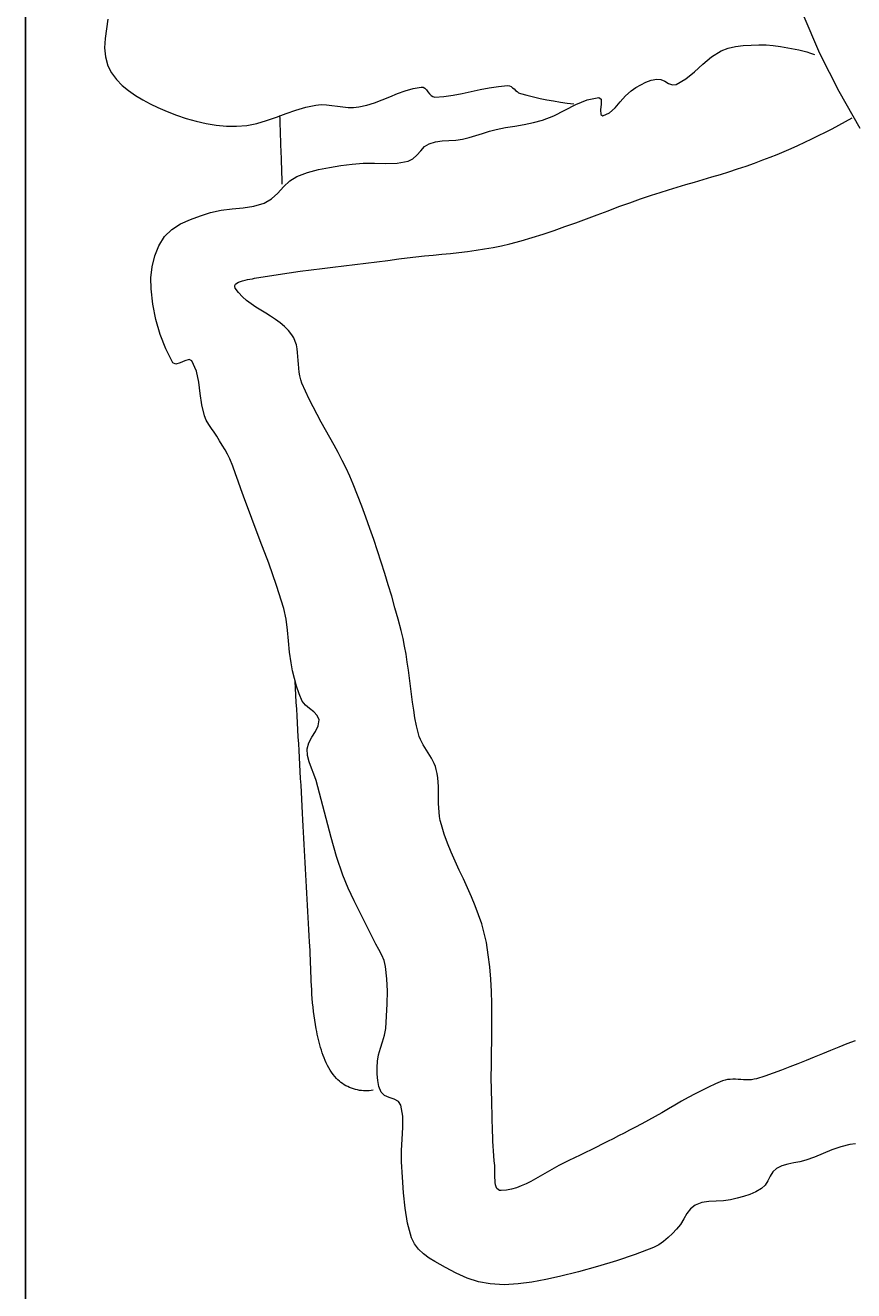
# Model space of a CAD drawing. Units: inches. Extents: x -15 to 423, y -713 to 71.
# Tile 5 of 24: x 34 to 57, y -195 to -159. Entities that reach past the tile are written whole.
import ezdxf

# ---------------------------------------------------------------- set-up
doc = ezdxf.new("R2010")
doc.units = ezdxf.units.IN
doc.header["$MEASUREMENT"] = 0
doc.layers.add('A-ANNO-DIMS', color=2, linetype='Continuous', lineweight=18)
doc.layers.add('A-FURN', color=9, linetype='Continuous', lineweight=13)
doc.styles.get("Standard").update_dxf_attribs({"font": 'arial.ttf'})
doc.dimstyles.get("Standard").update_dxf_attribs({"dimtxt": 0.18, "dimasz": 0.18, "dimexe": 0.18, "dimexo": 0.0625, "dimgap": 0.09, "dimtad": 0, "dimtih": 1, "dimtoh": 1, "dimdec": 0, "dimzin": 0, "dimdsep": 46, "dimlunit": 3, "dimtxsty": 'Standard', "dimcen": 0.09, "dimadec": 0, "dimazin": 0, "dimtfac": 1, "dimtdec": 0, "dimtofl": 0, "dimtmove": 0, "dimatfit": 3, "dimfxl": 1, "dimtolj": 1, "dimtzin": 0, "dimarcsym": 0})

# ---------------------------------------------------------------- blocks, each defined once
blk = doc.blocks.new('*D37')
at = {"layer": 'A-ANNO-DIMS', "color": 0, "lineweight": -2, "transparency": 16777216}
for p, q in [((34.081, -396.437), (34.081, 57.43)), ((34.261, 57.25), (47.648, 57.25)), ((61.698, 57.25), (48.31, 57.25)), ((61.878, -396.437), (61.878, 57.43))]:
    blk.add_line(p, q, dxfattribs=at)
at = {"layer": 'A-ANNO-DIMS', "color": 0, "transparency": 16777216}
for points in [[(34.261, 57.28), (34.261, 57.22), (34.081, 57.25)], [(61.698, 57.28), (61.698, 57.22), (61.878, 57.25)]]:
    blk.add_solid(points, dxfattribs=at)
at = {"layer": 'Defpoints', "color": 0, "transparency": 16777216}
for p in [(61.878, 57.25), (34.081, -396.5), (61.878, -396.5)]:
    blk.add_point(p, dxfattribs=at)
at = {"layer": 'A-ANNO-DIMS', "color": 0, "transparency": 16777216, "insert": (47.979, 57.25), "char_height": 0.18, "attachment_point": 5}
blk.add_mtext('\\A1;2\'-4"', dxfattribs=at)

msp = doc.modelspace()

# ---------------------------------------------------------------- linework, layer by layer
at = {"layer": 'A-FURN'}
for p, q in [((55.743, -158.982), (56.209, -160.068)), ((36.338, -159.391), (36.303, -159.656)), ((36.382, -159.123), (36.338, -159.391)), ((36.303, -159.656), (36.289, -159.918)), ((36.289, -159.918), (36.311, -160.173)), ((53.201, -160.167), (53.466, -160.003)), ((53.466, -160.003), (53.664, -159.928)), ((53.664, -159.928), (53.87, -159.88)), ((53.87, -159.88), (54.083, -159.853)), ((54.083, -159.853), (54.299, -159.84)), ((54.299, -159.84), (54.513, -159.834)), ((54.513, -159.834), (54.716, -159.837)), ((54.716, -159.837), (54.919, -159.855)), ((54.919, -159.855), (55.122, -159.883)), ((55.122, -159.883), (55.324, -159.917)), ((55.324, -159.917), (55.525, -159.953)), ((55.525, -159.953), (55.635, -159.975)), ((55.635, -159.975), (55.744, -160.001)), ((55.744, -160.001), (55.852, -160.031)), ((55.852, -160.031), (55.959, -160.066)), ((55.959, -160.066), (56.064, -160.105)), ((56.209, -160.068), (56.745, -161.125)), ((36.311, -160.173), (36.382, -160.419)), ((36.382, -160.419), (36.485, -160.619)), ((52.725, -160.585), (52.959, -160.37)), ((52.959, -160.37), (53.201, -160.167)), ((36.485, -160.619), (36.619, -160.8)), ((36.619, -160.8), (36.778, -160.964)), ((51.52, -160.822), (51.673, -160.788)), ((51.673, -160.788), (51.784, -160.801)), ((51.784, -160.801), (51.893, -160.852)), ((52.212, -160.94), (52.481, -160.784)), ((52.481, -160.784), (52.725, -160.585)), ((36.778, -160.964), (36.957, -161.112)), ((36.957, -161.112), (37.151, -161.247)), ((44.452, -161.194), (44.667, -161.116)), ((44.667, -161.116), (44.885, -161.052)), ((44.885, -161.052), (45.108, -161.01)), ((45.108, -161.01), (45.163, -161.016)), ((45.163, -161.016), (45.211, -161.045)), ((45.211, -161.045), (45.255, -161.09)), ((45.255, -161.09), (45.297, -161.143)), ((45.297, -161.143), (45.338, -161.196)), ((46.249, -161.191), (46.502, -161.137)), ((46.502, -161.137), (46.754, -161.082)), ((46.754, -161.082), (47.007, -161.032)), ((47.007, -161.032), (47.261, -160.993)), ((47.261, -160.993), (47.517, -160.972)), ((47.517, -160.972), (47.567, -160.978)), ((47.567, -160.978), (47.612, -160.998)), ((47.612, -160.998), (47.655, -161.029)), ((47.655, -161.029), (47.697, -161.065)), ((47.697, -161.065), (47.738, -161.103)), ((47.738, -161.103), (47.78, -161.139)), ((47.78, -161.139), (47.824, -161.17)), ((47.824, -161.17), (47.873, -161.19)), ((50.8, -161.256), (50.96, -161.115)), ((50.96, -161.115), (51.092, -161.028)), ((51.092, -161.028), (51.23, -160.946)), ((51.23, -160.946), (51.372, -160.876)), ((51.372, -160.876), (51.52, -160.822)), ((51.893, -160.852), (52.002, -160.912)), ((52.002, -160.912), (52.108, -160.95)), ((52.108, -160.95), (52.212, -160.94)), ((56.745, -161.125), (57.334, -162.155)), ((37.151, -161.247), (37.355, -161.369)), ((37.355, -161.369), (37.562, -161.479)), ((37.562, -161.479), (37.769, -161.58)), ((41.895, -161.573), (42.175, -161.514)), ((42.175, -161.514), (42.324, -161.501)), ((42.324, -161.501), (42.473, -161.506)), ((42.473, -161.506), (42.623, -161.521)), ((42.623, -161.521), (42.774, -161.543)), ((43.371, -161.567), (43.593, -161.517)), ((43.593, -161.517), (43.811, -161.448)), ((43.811, -161.448), (44.025, -161.367)), ((44.025, -161.367), (44.238, -161.28)), ((44.238, -161.28), (44.452, -161.194)), ((45.338, -161.196), (45.383, -161.244)), ((45.383, -161.244), (45.431, -161.277)), ((45.431, -161.277), (45.486, -161.289)), ((45.486, -161.289), (45.742, -161.274)), ((45.742, -161.274), (45.996, -161.239)), ((45.996, -161.239), (46.249, -161.191)), ((47.873, -161.19), (48.056, -161.239)), ((48.056, -161.239), (48.241, -161.284)), ((48.241, -161.284), (48.426, -161.326)), ((48.426, -161.326), (48.612, -161.365)), ((48.612, -161.365), (48.799, -161.4)), ((48.799, -161.4), (48.986, -161.431)), ((48.986, -161.431), (49.174, -161.459)), ((49.111, -161.652), (49.418, -161.494)), ((49.174, -161.459), (49.363, -161.483)), ((49.418, -161.494), (49.731, -161.367)), ((49.731, -161.367), (50.058, -161.301)), ((50.058, -161.301), (50.121, -161.353)), ((50.125, -161.486), (50.109, -161.645)), ((50.121, -161.353), (50.125, -161.486)), ((50.516, -161.594), (50.657, -161.426)), ((50.657, -161.426), (50.8, -161.256)), ((37.769, -161.58), (38.028, -161.695)), ((38.028, -161.695), (38.294, -161.798)), ((38.294, -161.798), (38.565, -161.889)), ((40.801, -161.943), (41.074, -161.849)), ((41.074, -161.849), (41.346, -161.749)), ((41.177, -161.902), (41.173, -161.806)), ((41.346, -161.749), (41.619, -161.654)), ((41.619, -161.654), (41.895, -161.573)), ((42.774, -161.543), (42.924, -161.564)), ((42.924, -161.564), (43.074, -161.579)), ((43.074, -161.579), (43.223, -161.582)), ((43.223, -161.582), (43.371, -161.567)), ((48.488, -161.937), (48.804, -161.81)), ((48.804, -161.81), (49.111, -161.652)), ((50.109, -161.645), (50.113, -161.773)), ((50.113, -161.773), (50.174, -161.813)), ((50.174, -161.813), (50.36, -161.732)), ((50.36, -161.732), (50.516, -161.594)), ((56.932, -161.974), (57.116, -161.871)), ((38.565, -161.889), (38.841, -161.966)), ((38.841, -161.966), (39.119, -162.027)), ((39.119, -162.027), (39.401, -162.071)), ((39.401, -162.071), (39.683, -162.097)), ((39.683, -162.097), (39.965, -162.103)), ((39.965, -162.103), (40.248, -162.079)), ((40.248, -162.079), (40.526, -162.023)), ((40.526, -162.023), (40.801, -161.943)), ((41.18, -161.997), (41.177, -161.902)), ((41.183, -162.093), (41.18, -161.997)), ((41.187, -162.189), (41.183, -162.093)), ((41.19, -162.285), (41.187, -162.189)), ((47.008, -162.245), (47.197, -162.195)), ((47.197, -162.195), (47.455, -162.142)), ((47.455, -162.142), (47.715, -162.098)), ((47.715, -162.098), (47.975, -162.055)), ((47.975, -162.055), (48.234, -162.004)), ((48.234, -162.004), (48.488, -161.937)), ((56.371, -162.27), (56.559, -162.173)), ((56.559, -162.173), (56.746, -162.075)), ((56.746, -162.075), (56.932, -161.974)), ((41.193, -162.38), (41.19, -162.285)), ((41.197, -162.476), (41.193, -162.38)), ((41.2, -162.572), (41.197, -162.476)), ((41.203, -162.667), (41.2, -162.572)), ((45.332, -162.59), (45.51, -162.539)), ((45.51, -162.539), (45.694, -162.514)), ((45.694, -162.514), (45.882, -162.503)), ((45.882, -162.503), (46.071, -162.492)), ((46.071, -162.492), (46.256, -162.465)), ((46.256, -162.465), (46.446, -162.418)), ((46.446, -162.418), (46.634, -162.362)), ((46.634, -162.362), (46.82, -162.303)), ((46.82, -162.303), (47.008, -162.245)), ((55.607, -162.636), (55.8, -162.548)), ((55.8, -162.548), (55.991, -162.457)), ((55.991, -162.457), (56.181, -162.365)), ((56.181, -162.365), (56.371, -162.27)), ((41.207, -162.763), (41.203, -162.667)), ((41.21, -162.859), (41.207, -162.763)), ((41.214, -162.954), (41.21, -162.859)), ((44.879, -163.012), (44.991, -162.906)), ((44.991, -162.906), (45.095, -162.785)), ((45.095, -162.785), (45.204, -162.672)), ((45.204, -162.672), (45.332, -162.59)), ((54.829, -162.967), (55.025, -162.887)), ((55.025, -162.887), (55.22, -162.806)), ((55.22, -162.806), (55.414, -162.722)), ((55.414, -162.722), (55.607, -162.636)), ((41.217, -163.05), (41.214, -162.954)), ((41.22, -163.146), (41.217, -163.05)), ((41.224, -163.241), (41.22, -163.146)), ((41.227, -163.337), (41.224, -163.241)), ((42.245, -163.31), (42.556, -163.249)), ((42.556, -163.249), (42.87, -163.201)), ((42.87, -163.201), (43.183, -163.158)), ((43.183, -163.158), (43.496, -163.135)), ((43.496, -163.135), (43.812, -163.137)), ((43.812, -163.137), (44.127, -163.143)), ((44.127, -163.143), (44.44, -163.131)), ((44.44, -163.131), (44.747, -163.078)), ((44.747, -163.078), (44.879, -163.012)), ((53.924, -163.294), (54.161, -163.215)), ((54.161, -163.215), (54.397, -163.131)), ((54.397, -163.131), (54.632, -163.044)), ((54.632, -163.044), (54.829, -162.967)), ((41.23, -163.433), (41.227, -163.337)), ((41.234, -163.528), (41.23, -163.433)), ((41.237, -163.624), (41.234, -163.528)), ((41.24, -163.72), (41.237, -163.624)), ((41.277, -163.791), (41.45, -163.628)), ((41.45, -163.628), (41.647, -163.504)), ((41.647, -163.504), (41.941, -163.393)), ((41.941, -163.393), (42.245, -163.31)), ((52.724, -163.659), (52.965, -163.588)), ((52.965, -163.588), (53.205, -163.517)), ((53.205, -163.517), (53.446, -163.445)), ((53.446, -163.445), (53.685, -163.371)), ((53.685, -163.371), (53.924, -163.294)), ((40.937, -164.127), (41.111, -163.966)), ((41.111, -163.966), (41.277, -163.791)), ((51.525, -164.026), (51.764, -163.948)), ((51.764, -163.948), (52.003, -163.874)), ((52.003, -163.874), (52.243, -163.801)), ((52.243, -163.801), (52.484, -163.73)), ((52.484, -163.73), (52.724, -163.659)), ((40.148, -164.378), (40.449, -164.334)), ((40.449, -164.334), (40.738, -164.247)), ((40.738, -164.247), (40.937, -164.127)), ((50.618, -164.345), (50.919, -164.236)), ((50.919, -164.236), (51.222, -164.129)), ((51.222, -164.129), (51.525, -164.026)), ((38.678, -164.703), (38.961, -164.602)), ((38.961, -164.602), (39.241, -164.51)), ((39.241, -164.51), (39.537, -164.439)), ((39.537, -164.439), (39.841, -164.404)), ((39.841, -164.404), (40.148, -164.378)), ((49.414, -164.793), (49.715, -164.682)), ((49.715, -164.682), (50.016, -164.57)), ((50.016, -164.57), (50.317, -164.457)), ((50.317, -164.457), (50.618, -164.345)), ((37.96, -165.18), (38.163, -164.979)), ((38.163, -164.979), (38.408, -164.824)), ((38.408, -164.824), (38.678, -164.703)), ((48.506, -165.109), (48.81, -165.008)), ((48.81, -165.008), (49.112, -164.902)), ((49.112, -164.902), (49.414, -164.793)), ((37.8, -165.434), (37.96, -165.18)), ((47.349, -165.433), (47.583, -165.378)), ((47.583, -165.378), (47.893, -165.295)), ((47.893, -165.295), (48.2, -165.206)), ((48.2, -165.206), (48.506, -165.109)), ((37.613, -166.018), (37.685, -165.717)), ((37.685, -165.717), (37.8, -165.434)), ((44.722, -165.773), (44.962, -165.746)), ((44.962, -165.746), (45.202, -165.72)), ((45.202, -165.72), (45.442, -165.696)), ((45.442, -165.696), (45.682, -165.672)), ((45.682, -165.672), (45.922, -165.647)), ((45.922, -165.647), (46.162, -165.621)), ((46.162, -165.621), (46.401, -165.592)), ((46.401, -165.592), (46.639, -165.559)), ((46.639, -165.559), (46.877, -165.523)), ((46.877, -165.523), (47.114, -165.481)), ((47.114, -165.481), (47.349, -165.433)), ((37.58, -166.326), (37.613, -166.018)), ((41.737, -166.145), (42.041, -166.105)), ((42.041, -166.105), (42.347, -166.066)), ((42.347, -166.066), (42.652, -166.029)), ((42.652, -166.029), (42.957, -165.992)), ((42.957, -165.992), (43.263, -165.956)), ((43.263, -165.956), (43.568, -165.919)), ((43.568, -165.919), (43.874, -165.882)), ((43.874, -165.882), (44.179, -165.844)), ((44.179, -165.844), (44.484, -165.803)), ((44.484, -165.803), (44.722, -165.773)), ((37.583, -166.631), (37.58, -166.326)), ((39.971, -166.476), (40.017, -166.451)), ((40.017, -166.451), (40.072, -166.429)), ((40.072, -166.429), (40.134, -166.409)), ((40.134, -166.409), (40.201, -166.392)), ((40.201, -166.392), (40.27, -166.377)), ((40.27, -166.377), (40.339, -166.364)), ((40.339, -166.364), (40.406, -166.352)), ((40.406, -166.352), (40.467, -166.342)), ((40.467, -166.342), (40.521, -166.332)), ((40.521, -166.332), (40.824, -166.281)), ((40.824, -166.281), (41.128, -166.232)), ((41.128, -166.232), (41.432, -166.187)), ((41.432, -166.187), (41.737, -166.145)), ((37.63, -167.06), (37.583, -166.631)), ((39.915, -166.574), (39.918, -166.538)), ((39.931, -166.615), (39.915, -166.574)), ((39.918, -166.538), (39.937, -166.505)), ((40.022, -166.741), (39.931, -166.615)), ((39.937, -166.505), (39.971, -166.476)), ((40.127, -166.855), (40.022, -166.741)), ((37.715, -167.487), (37.63, -167.06)), ((40.244, -166.959), (40.127, -166.855)), ((40.369, -167.054), (40.244, -166.959)), ((40.502, -167.144), (40.369, -167.054)), ((40.639, -167.23), (40.502, -167.144)), ((37.837, -167.906), (37.715, -167.487)), ((40.777, -167.315), (40.639, -167.23)), ((40.915, -167.4), (40.777, -167.315)), ((41.049, -167.488), (40.915, -167.4)), ((41.179, -167.582), (41.049, -167.488)), ((41.299, -167.682), (41.179, -167.582)), ((41.41, -167.793), (41.299, -167.682)), ((41.507, -167.915), (41.41, -167.793)), ((37.995, -168.31), (37.837, -167.906)), ((41.561, -168.005), (41.507, -167.915)), ((41.602, -168.1), (41.561, -168.005)), ((41.632, -168.2), (41.602, -168.1)), ((41.653, -168.303), (41.632, -168.2)), ((38.19, -168.696), (37.995, -168.31)), ((41.667, -168.41), (41.653, -168.303)), ((41.677, -168.518), (41.667, -168.41)), ((41.684, -168.628), (41.677, -168.518)), ((38.27, -168.735), (38.19, -168.696)), ((38.39, -168.7), (38.27, -168.735)), ((38.522, -168.639), (38.39, -168.7)), ((38.642, -168.603), (38.522, -168.639)), ((38.724, -168.642), (38.642, -168.603)), ((38.847, -168.927), (38.724, -168.642)), ((38.915, -169.234), (38.847, -168.927)), ((41.691, -168.738), (41.684, -168.628)), ((41.699, -168.848), (41.691, -168.738)), ((41.71, -168.957), (41.699, -168.848)), ((38.955, -169.552), (38.915, -169.234)), ((41.728, -169.063), (41.71, -168.957)), ((41.753, -169.167), (41.728, -169.063)), ((41.787, -169.267), (41.753, -169.167)), ((41.883, -169.49), (41.787, -169.267)), ((38.997, -169.87), (38.955, -169.552)), ((41.987, -169.709), (41.883, -169.49)), ((39.07, -170.178), (38.997, -169.87)), ((42.096, -169.925), (41.987, -169.709)), ((42.209, -170.139), (42.096, -169.925)), ((39.122, -170.3), (39.07, -170.178)), ((39.189, -170.414), (39.122, -170.3)), ((42.326, -170.352), (42.209, -170.139)), ((39.264, -170.525), (39.189, -170.414)), ((39.341, -170.634), (39.264, -170.525)), ((39.414, -170.746), (39.341, -170.634)), ((42.445, -170.564), (42.326, -170.352)), ((42.564, -170.776), (42.445, -170.564)), ((39.49, -170.871), (39.414, -170.746)), ((39.567, -170.994), (39.49, -170.871)), ((39.644, -171.119), (39.567, -170.994)), ((42.682, -170.988), (42.564, -170.776)), ((42.798, -171.201), (42.682, -170.988)), ((39.715, -171.245), (39.644, -171.119)), ((39.779, -171.376), (39.715, -171.245)), ((39.864, -171.58), (39.779, -171.376)), ((42.911, -171.416), (42.798, -171.201)), ((39.94, -171.788), (39.864, -171.58)), ((43.019, -171.632), (42.911, -171.416)), ((43.121, -171.852), (43.019, -171.632)), ((40.011, -171.998), (39.94, -171.788)), ((40.082, -172.208), (40.011, -171.998)), ((43.215, -172.075), (43.121, -171.852)), ((43.336, -172.383), (43.215, -172.075)), ((40.155, -172.417), (40.082, -172.208)), ((40.387, -173.04), (40.155, -172.417)), ((43.455, -172.692), (43.336, -172.383)), ((43.57, -173.002), (43.455, -172.692)), ((40.626, -173.66), (40.387, -173.04)), ((43.681, -173.313), (43.57, -173.002)), ((43.79, -173.626), (43.681, -173.313)), ((40.861, -174.282), (40.626, -173.66)), ((43.895, -173.94), (43.79, -173.626)), ((43.998, -174.255), (43.895, -173.94)), ((41.083, -174.907), (40.861, -174.282)), ((44.097, -174.57), (43.998, -174.255)), ((44.194, -174.887), (44.097, -174.57)), ((41.281, -175.541), (41.083, -174.907)), ((44.287, -175.205), (44.194, -174.887)), ((44.378, -175.523), (44.287, -175.205)), ((41.346, -175.839), (41.281, -175.541)), ((44.465, -175.842), (44.378, -175.523)), ((41.384, -176.144), (41.346, -175.839)), ((44.55, -176.162), (44.465, -175.842)), ((41.409, -176.45), (41.384, -176.144)), ((44.603, -176.379), (44.55, -176.162)), ((41.437, -176.757), (41.409, -176.45)), ((44.648, -176.598), (44.603, -176.379)), ((44.687, -176.819), (44.648, -176.598)), ((41.483, -177.06), (41.437, -176.757)), ((44.721, -177.04), (44.687, -176.819)), ((41.528, -177.278), (41.483, -177.06)), ((41.578, -177.496), (41.528, -177.278)), ((44.752, -177.263), (44.721, -177.04)), ((44.78, -177.485), (44.752, -177.263)), ((41.637, -177.71), (41.578, -177.496)), ((41.609, -177.766), (41.598, -177.572)), ((41.709, -177.92), (41.637, -177.71)), ((44.808, -177.708), (44.78, -177.485)), ((44.836, -177.931), (44.808, -177.708)), ((41.62, -177.959), (41.609, -177.766)), ((41.631, -178.152), (41.62, -177.959)), ((41.797, -178.124), (41.709, -177.92)), ((44.866, -178.153), (44.836, -177.931)), ((41.642, -178.346), (41.631, -178.152)), ((41.653, -178.539), (41.642, -178.346)), ((41.883, -178.236), (41.797, -178.124)), ((41.999, -178.332), (41.883, -178.236)), ((42.119, -178.423), (41.999, -178.332)), ((42.215, -178.524), (42.119, -178.423)), ((44.9, -178.375), (44.866, -178.153)), ((44.937, -178.596), (44.9, -178.375)), ((41.664, -178.732), (41.653, -178.539)), ((41.675, -178.926), (41.664, -178.732)), ((42.263, -178.648), (42.215, -178.524)), ((42.241, -178.816), (42.263, -178.648)), ((44.981, -178.815), (44.937, -178.596)), ((41.686, -179.119), (41.675, -178.926)), ((41.697, -179.312), (41.686, -179.119)), ((41.975, -179.29), (42.064, -179.131)), ((42.064, -179.131), (42.163, -178.975)), ((42.163, -178.975), (42.241, -178.816)), ((45.032, -179.033), (44.981, -178.815)), ((45.057, -179.115), (45.032, -179.033)), ((45.089, -179.194), (45.057, -179.115)), ((41.708, -179.506), (41.697, -179.312)), ((41.719, -179.699), (41.708, -179.506)), ((41.933, -179.459), (41.975, -179.29)), ((41.945, -179.639), (41.933, -179.459)), ((45.126, -179.271), (45.089, -179.194)), ((45.167, -179.347), (45.126, -179.271)), ((45.212, -179.421), (45.167, -179.347)), ((45.258, -179.495), (45.212, -179.421)), ((45.305, -179.569), (45.258, -179.495)), ((41.73, -179.892), (41.719, -179.699)), ((41.99, -179.816), (41.945, -179.639)), ((42.053, -179.99), (41.99, -179.816)), ((45.351, -179.642), (45.305, -179.569)), ((45.396, -179.717), (45.351, -179.642)), ((45.437, -179.792), (45.396, -179.717)), ((45.474, -179.869), (45.437, -179.792)), ((41.74, -180.086), (41.73, -179.892)), ((41.751, -180.279), (41.74, -180.086)), ((42.122, -180.164), (42.053, -179.99)), ((42.181, -180.339), (42.122, -180.164)), ((45.506, -179.949), (45.474, -179.869)), ((45.53, -180.03), (45.506, -179.949)), ((45.555, -180.147), (45.53, -180.03)), ((45.572, -180.264), (45.555, -180.147)), ((41.762, -180.472), (41.751, -180.279)), ((41.773, -180.666), (41.762, -180.472)), ((42.323, -180.868), (42.181, -180.339)), ((45.583, -180.383), (45.572, -180.264)), ((45.589, -180.502), (45.583, -180.383)), ((45.592, -180.622), (45.589, -180.502)), ((41.784, -180.859), (41.773, -180.666)), ((41.794, -181.052), (41.784, -180.859)), ((42.46, -181.4), (42.323, -180.868)), ((45.594, -180.743), (45.592, -180.622)), ((45.594, -180.863), (45.594, -180.743)), ((45.596, -180.983), (45.594, -180.863)), ((41.805, -181.246), (41.794, -181.052)), ((41.816, -181.439), (41.805, -181.246)), ((45.6, -181.103), (45.596, -180.983)), ((45.609, -181.222), (45.6, -181.103)), ((45.622, -181.34), (45.609, -181.222)), ((41.825, -181.609), (41.816, -181.439)), ((41.835, -181.778), (41.825, -181.609)), ((42.6, -181.93), (42.46, -181.4)), ((45.642, -181.457), (45.622, -181.34)), ((45.671, -181.572), (45.642, -181.457)), ((45.752, -181.83), (45.671, -181.572)), ((41.844, -181.948), (41.835, -181.778)), ((41.853, -182.118), (41.844, -181.948)), ((42.752, -182.457), (42.6, -181.93)), ((45.846, -182.084), (45.752, -181.83)), ((41.861, -182.288), (41.853, -182.118)), ((41.87, -182.457), (41.861, -182.288)), ((45.948, -182.335), (45.846, -182.084)), ((41.879, -182.627), (41.87, -182.457)), ((41.888, -182.797), (41.879, -182.627)), ((42.924, -182.977), (42.752, -182.457)), ((46.057, -182.585), (45.948, -182.335)), ((46.17, -182.833), (46.057, -182.585)), ((41.897, -182.966), (41.888, -182.797)), ((41.906, -183.136), (41.897, -182.966)), ((43.071, -183.341), (42.924, -182.977)), ((46.284, -183.081), (46.17, -182.833)), ((41.915, -183.306), (41.906, -183.136)), ((41.924, -183.476), (41.915, -183.306)), ((43.238, -183.696), (43.071, -183.341)), ((46.398, -183.328), (46.284, -183.081)), ((46.508, -183.577), (46.398, -183.328)), ((41.933, -183.645), (41.924, -183.476)), ((41.942, -183.815), (41.933, -183.645)), ((43.417, -184.047), (43.238, -183.696)), ((46.613, -183.827), (46.508, -183.577)), ((41.951, -183.985), (41.942, -183.815)), ((41.961, -184.154), (41.951, -183.985)), ((43.597, -184.396), (43.417, -184.047)), ((46.709, -184.079), (46.613, -183.827)), ((46.795, -184.334), (46.709, -184.079)), ((41.971, -184.324), (41.961, -184.154)), ((41.981, -184.494), (41.971, -184.324)), ((43.771, -184.749), (43.597, -184.396)), ((46.868, -184.594), (46.795, -184.334)), ((41.991, -184.663), (41.981, -184.494)), ((42.002, -184.833), (41.991, -184.663)), ((43.849, -184.901), (43.771, -184.749)), ((46.925, -184.857), (46.868, -184.594)), ((42.009, -184.954), (42.002, -184.833)), ((42.015, -185.076), (42.009, -184.954)), ((42.02, -185.198), (42.015, -185.076)), ((43.934, -185.051), (43.849, -184.901)), ((44.014, -185.203), (43.934, -185.051)), ((46.978, -185.195), (46.925, -184.857)), ((42.025, -185.32), (42.02, -185.198)), ((42.03, -185.441), (42.025, -185.32)), ((42.034, -185.563), (42.03, -185.441)), ((44.08, -185.359), (44.014, -185.203)), ((44.119, -185.523), (44.08, -185.359)), ((47.018, -185.533), (46.978, -185.195)), ((42.038, -185.685), (42.034, -185.563)), ((42.043, -185.807), (42.038, -185.685)), ((42.048, -185.929), (42.043, -185.807)), ((44.155, -185.867), (44.119, -185.523)), ((47.047, -185.874), (47.018, -185.533)), ((42.053, -186.051), (42.048, -185.929)), ((42.06, -186.173), (42.053, -186.051)), ((42.067, -186.294), (42.06, -186.173)), ((44.168, -186.213), (44.155, -185.867)), ((47.065, -186.215), (47.047, -185.874)), ((42.075, -186.416), (42.067, -186.294)), ((42.085, -186.537), (42.075, -186.416)), ((42.097, -186.658), (42.085, -186.537)), ((44.147, -186.907), (44.164, -186.56)), ((44.164, -186.56), (44.168, -186.213)), ((47.074, -186.557), (47.065, -186.215)), ((47.078, -186.9), (47.074, -186.557)), ((42.11, -186.779), (42.097, -186.658)), ((42.125, -186.899), (42.11, -186.779)), ((42.142, -187.019), (42.125, -186.899)), ((44.12, -187.253), (44.147, -186.907)), ((47.077, -187.243), (47.078, -186.9)), ((42.162, -187.139), (42.142, -187.019)), ((42.184, -187.259), (42.162, -187.139)), ((42.199, -187.333), (42.184, -187.259)), ((44.089, -187.437), (44.12, -187.253)), ((47.073, -187.586), (47.077, -187.243)), ((42.215, -187.407), (42.199, -187.333)), ((42.231, -187.481), (42.215, -187.407)), ((42.248, -187.556), (42.231, -187.481)), ((42.266, -187.631), (42.248, -187.556)), ((43.976, -187.799), (44.036, -187.619)), ((44.036, -187.619), (44.089, -187.437)), ((47.068, -187.93), (47.073, -187.586)), ((57.201, -187.59), (56.972, -187.679)), ((42.286, -187.705), (42.266, -187.631)), ((42.306, -187.779), (42.286, -187.705)), ((42.329, -187.853), (42.306, -187.779)), ((42.352, -187.926), (42.329, -187.853)), ((42.378, -187.998), (42.352, -187.926)), ((43.924, -187.98), (43.976, -187.799)), ((47.064, -188.274), (47.068, -187.93)), ((56.289, -187.955), (56.062, -188.049)), ((56.516, -187.862), (56.289, -187.955)), ((56.744, -187.769), (56.516, -187.862)), ((56.972, -187.679), (56.744, -187.769)), ((42.405, -188.07), (42.378, -187.998)), ((42.434, -188.14), (42.405, -188.07)), ((42.466, -188.209), (42.434, -188.14)), ((42.499, -188.277), (42.466, -188.209)), ((42.535, -188.343), (42.499, -188.277)), ((43.885, -188.341), (43.895, -188.165)), ((43.895, -188.165), (43.924, -187.98)), ((47.062, -188.617), (47.064, -188.274)), ((55.378, -188.323), (55.148, -188.411)), ((55.606, -188.233), (55.378, -188.323)), ((55.834, -188.142), (55.606, -188.233)), ((56.062, -188.049), (55.834, -188.142)), ((42.573, -188.408), (42.535, -188.343)), ((42.614, -188.47), (42.573, -188.408)), ((42.658, -188.531), (42.614, -188.47)), ((42.704, -188.589), (42.658, -188.531)), ((42.754, -188.645), (42.704, -188.589)), ((42.791, -188.684), (42.754, -188.645)), ((43.884, -188.519), (43.885, -188.341)), ((43.898, -188.696), (43.884, -188.519)), ((47.065, -188.96), (47.062, -188.617)), ((53.645, -188.676), (53.575, -188.69)), ((53.717, -188.668), (53.645, -188.676)), ((53.79, -188.665), (53.717, -188.668)), ((53.864, -188.666), (53.79, -188.665)), ((53.939, -188.669), (53.864, -188.666)), ((54.013, -188.674), (53.939, -188.669)), ((54.088, -188.679), (54.013, -188.674)), ((54.31, -188.677), (54.237, -188.681)), ((54.382, -188.666), (54.31, -188.677)), ((54.452, -188.649), (54.382, -188.666)), ((54.686, -188.574), (54.452, -188.649)), ((54.918, -188.494), (54.686, -188.574)), ((55.148, -188.411), (54.918, -188.494)), ((42.831, -188.72), (42.791, -188.684)), ((42.874, -188.754), (42.831, -188.72)), ((42.919, -188.786), (42.874, -188.754)), ((42.966, -188.817), (42.919, -188.786)), ((43.014, -188.845), (42.966, -188.817)), ((43.064, -188.87), (43.014, -188.845)), ((43.116, -188.894), (43.064, -188.87)), ((43.168, -188.915), (43.116, -188.894)), ((43.222, -188.933), (43.168, -188.915)), ((43.277, -188.949), (43.222, -188.933)), ((43.332, -188.963), (43.277, -188.949)), ((43.387, -188.974), (43.332, -188.963)), ((43.443, -188.982), (43.387, -188.974)), ((43.499, -188.987), (43.443, -188.982)), ((43.554, -188.99), (43.499, -188.987)), ((43.61, -188.99), (43.554, -188.99)), ((43.664, -188.986), (43.61, -188.99)), ((43.718, -188.98), (43.664, -188.986)), ((43.771, -188.971), (43.718, -188.98)), ((43.934, -188.867), (43.898, -188.696)), ((43.999, -189.027), (43.934, -188.867)), ((44.088, -189.118), (43.999, -189.027)), ((47.074, -189.302), (47.065, -188.96)), ((52.927, -188.977), (52.738, -189.074)), ((53.118, -188.884), (52.927, -188.977)), ((53.311, -188.796), (53.118, -188.884)), ((53.506, -188.713), (53.311, -188.796)), ((53.575, -188.69), (53.506, -188.713)), ((54.163, -188.681), (54.088, -188.679)), ((54.237, -188.681), (54.163, -188.681)), ((44.217, -189.176), (44.088, -189.118)), ((44.355, -189.224), (44.217, -189.176)), ((44.473, -189.286), (44.355, -189.224)), ((44.543, -189.385), (44.473, -189.286)), ((47.079, -189.438), (47.074, -189.302)), ((52.18, -189.384), (51.996, -189.49)), ((52.365, -189.278), (52.18, -189.384)), ((52.551, -189.175), (52.365, -189.278)), ((52.738, -189.074), (52.551, -189.175)), ((44.597, -189.694), (44.543, -189.385)), ((44.601, -190.01), (44.597, -189.694)), ((47.083, -189.575), (47.079, -189.438)), ((47.087, -189.711), (47.083, -189.575)), ((47.09, -189.847), (47.087, -189.711)), ((51.626, -189.702), (51.441, -189.807)), ((51.811, -189.596), (51.626, -189.702)), ((51.996, -189.49), (51.811, -189.596)), ((44.579, -190.331), (44.601, -190.01)), ((47.094, -189.984), (47.09, -189.847)), ((47.099, -190.12), (47.094, -189.984)), ((50.914, -190.087), (50.762, -190.165)), ((51.066, -190.008), (50.914, -190.087)), ((51.254, -189.909), (51.066, -190.008)), ((51.441, -189.807), (51.254, -189.909)), ((44.557, -190.652), (44.579, -190.331)), ((47.103, -190.256), (47.099, -190.12)), ((47.109, -190.392), (47.103, -190.256)), ((47.116, -190.528), (47.109, -190.392)), ((50.303, -190.399), (50.15, -190.477)), ((50.456, -190.322), (50.303, -190.399)), ((50.609, -190.244), (50.456, -190.322)), ((50.762, -190.165), (50.609, -190.244)), ((44.561, -190.97), (44.557, -190.652)), ((47.124, -190.664), (47.116, -190.528)), ((47.133, -190.8), (47.124, -190.664)), ((49.536, -190.782), (49.382, -190.857)), ((49.69, -190.706), (49.536, -190.782)), ((49.844, -190.63), (49.69, -190.706)), ((49.997, -190.554), (49.844, -190.63)), ((50.15, -190.477), (49.997, -190.554)), ((56.312, -190.732), (56.071, -190.832)), ((56.554, -190.632), (56.312, -190.732)), ((56.799, -190.544), (56.554, -190.632)), ((57.051, -190.481), (56.799, -190.544)), ((57.206, -190.469), (57.051, -190.481)), ((44.59, -191.397), (44.561, -190.97)), ((47.145, -190.936), (47.133, -190.8)), ((47.158, -191.072), (47.145, -190.936)), ((47.163, -191.13), (47.158, -191.072)), ((47.164, -191.195), (47.163, -191.13)), ((48.811, -191.141), (48.682, -191.215)), ((48.941, -191.07), (48.811, -191.141)), ((49.072, -191.004), (48.941, -191.07)), ((49.227, -190.931), (49.072, -191.004)), ((49.382, -190.857), (49.227, -190.931)), ((55.158, -191.074), (55.007, -191.148)), ((55.321, -191.028), (55.158, -191.074)), ((55.49, -190.996), (55.321, -191.028)), ((55.66, -190.965), (55.49, -190.996)), ((55.826, -190.922), (55.66, -190.965)), ((56.071, -190.832), (55.826, -190.922)), ((44.618, -191.826), (44.59, -191.397)), ((47.164, -191.264), (47.164, -191.195)), ((47.164, -191.336), (47.164, -191.264)), ((47.164, -191.408), (47.164, -191.336)), ((47.167, -191.478), (47.164, -191.408)), ((47.172, -191.545), (47.167, -191.478)), ((48.294, -191.442), (48.163, -191.514)), ((48.424, -191.368), (48.294, -191.442)), ((48.553, -191.291), (48.424, -191.368)), ((48.682, -191.215), (48.553, -191.291)), ((54.763, -191.494), (54.688, -191.617)), ((54.83, -191.364), (54.763, -191.494)), ((54.907, -191.243), (54.83, -191.364)), ((55.007, -191.148), (54.907, -191.243)), ((44.66, -192.253), (44.618, -191.826)), ((47.183, -191.607), (47.172, -191.545)), ((47.198, -191.661), (47.183, -191.607)), ((47.221, -191.706), (47.198, -191.661)), ((47.251, -191.74), (47.221, -191.706)), ((47.29, -191.761), (47.251, -191.74)), ((47.34, -191.767), (47.29, -191.761)), ((47.484, -191.755), (47.34, -191.767)), ((47.625, -191.728), (47.484, -191.755)), ((47.762, -191.688), (47.625, -191.728)), ((47.898, -191.638), (47.762, -191.688)), ((48.031, -191.579), (47.898, -191.638)), ((48.163, -191.514), (48.031, -191.579)), ((54.432, -191.806), (54.264, -191.876)), ((54.589, -191.714), (54.432, -191.806)), ((54.688, -191.617), (54.589, -191.714)), ((52.746, -192.171), (52.616, -192.274)), ((52.93, -192.103), (52.746, -192.171)), ((53.126, -192.074), (52.93, -192.103)), ((53.329, -192.064), (53.126, -192.074)), ((53.533, -192.054), (53.329, -192.064)), ((53.731, -192.024), (53.533, -192.054)), ((53.91, -191.98), (53.731, -192.024)), ((54.088, -191.933), (53.91, -191.98)), ((54.264, -191.876), (54.088, -191.933)), ((44.729, -192.674), (44.66, -192.253)), ((52.513, -192.408), (52.424, -192.558)), ((52.616, -192.274), (52.513, -192.408)), ((44.839, -193.085), (44.729, -192.674)), ((52.227, -192.843), (52.11, -192.961)), ((52.333, -192.709), (52.227, -192.843)), ((52.424, -192.558), (52.333, -192.709)), ((44.919, -193.252), (44.839, -193.085)), ((45.035, -193.4), (44.919, -193.252)), ((51.862, -193.185), (51.727, -193.279)), ((51.989, -193.077), (51.862, -193.185)), ((52.11, -192.961), (51.989, -193.077)), ((45.176, -193.532), (45.035, -193.4)), ((45.332, -193.647), (45.176, -193.532)), ((51.069, -193.549), (50.55, -193.726)), ((51.58, -193.353), (51.069, -193.549)), ((51.727, -193.279), (51.58, -193.353)), ((45.493, -193.748), (45.332, -193.647)), ((45.784, -193.914), (45.493, -193.748)), ((46.083, -194.069), (45.784, -193.914)), ((50.026, -193.887), (49.496, -194.031)), ((50.55, -193.726), (50.026, -193.887)), ((46.391, -194.204), (46.083, -194.069)), ((46.707, -194.307), (46.391, -194.204)), ((47.033, -194.37), (46.707, -194.307)), ((48.196, -194.316), (47.808, -194.369)), ((48.582, -194.242), (48.196, -194.316)), ((48.964, -194.158), (48.582, -194.242)), ((49.496, -194.031), (48.964, -194.158)), ((47.42, -194.391), (47.033, -194.37)), ((47.808, -194.369), (47.42, -194.391))]:
    msp.add_line(p, q, dxfattribs=at)

# ---------------------------------------------------------------- dimensions: what is measured, and where the dimension line sits
at = {"layer": 'A-ANNO-DIMS'}
dim = msp.add_linear_dim(base=(61.878, 57.25), p1=(34.081, -396.5), p2=(61.878, -396.5), dimstyle='Standard', override={"dimdec": 1, "dimlfac": 1, "dimrnd": 0, "dimzin": 1, "dimdsep": 46, "dimlunit": 4, "dimfrac": 2}, dxfattribs=at)
dim.commit()
dim.dimension.update_dxf_attribs({"geometry": '*D37', "text_midpoint": (47.979, 57.25)})

doc.saveas('drawing.dxf')
